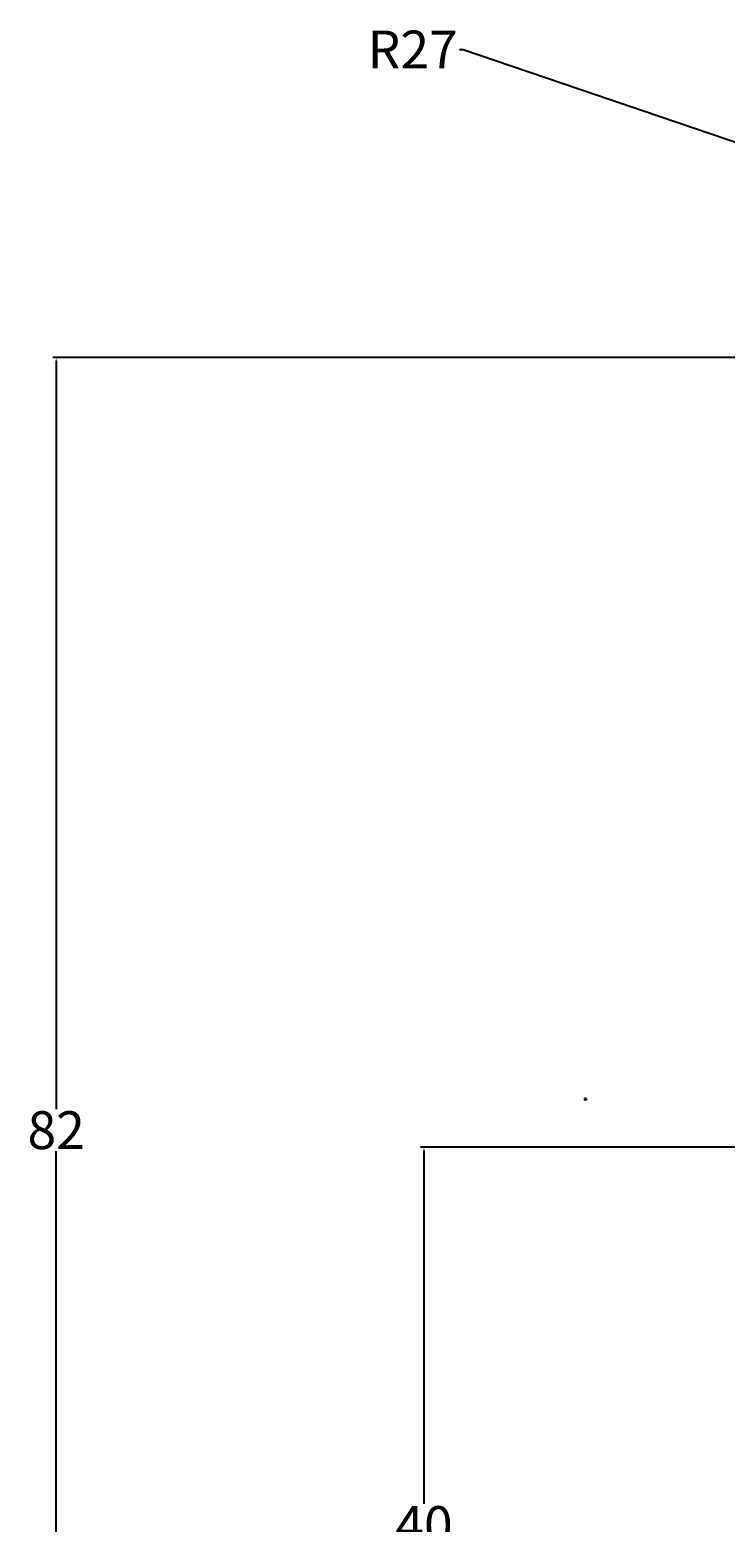
# Model space of a CAD drawing. Units: millimetres. Extents: x -60 to 113, y -37 to 126.
# Tile 6 of 17: x -60 to -23, y 27 to 106. Entities that reach past the tile are written whole.
import ezdxf

# ---------------------------------------------------------------- set-up
doc = ezdxf.new("R2010")
doc.units = ezdxf.units.MM
doc.header["$MEASUREMENT"] = 0
doc.layers.add('M-DIMS', color=2, linetype='Continuous', lineweight=25)
doc.styles.get("Standard").update_dxf_attribs({"font": 'arial.ttf'})
doc.dimstyles.get("Standard").update_dxf_attribs({"dimtxt": 0.18, "dimasz": 0.18, "dimexe": 0.18, "dimexo": 0.0625, "dimgap": 0.09, "dimtad": 0, "dimtih": 1, "dimtoh": 1, "dimdec": 4, "dimzin": 0, "dimdsep": 46, "dimtxsty": 'Standard', "dimcen": 0.09, "dimadec": 0, "dimazin": 0, "dimtfac": 1, "dimtdec": 4, "dimtofl": 0, "dimtmove": 0, "dimatfit": 3, "dimfxl": 1, "dimtolj": 1, "dimtzin": 0, "dimarcsym": 0})

# ---------------------------------------------------------------- blocks, each defined once
blk = doc.blocks.new('*D4')
at = {"layer": 'Defpoints', "color": 0, "transparency": 16777216}
for p in [(-14.94, 97.225), (10.622, 88.533)]:
    blk.add_point(p, dxfattribs=at)
at = {"layer": 'M-DIMS', "color": 0, "lineweight": -2, "transparency": 16777216}
for p, q in [((-37.421, 104.807), (-37.241, 104.807)), ((-37.241, 104.807), (-15.111, 97.283)), ((10.532, 88.533), (10.712, 88.533)), ((10.622, 88.443), (10.622, 88.623))]:
    blk.add_line(p, q, dxfattribs=at)
at = {"layer": 'M-DIMS', "color": 0, "transparency": 16777216}
blk.add_solid([(-15.101, 97.311), (-15.12, 97.254), (-14.94, 97.225)], dxfattribs=at)
at = {"layer": 'M-DIMS', "color": 0, "transparency": 16777216, "insert": (-39.9, 104.807), "char_height": 0.18, "attachment_point": 5}
blk.add_mtext('\\A1;{\\H11.11111x;R27}', dxfattribs=at)
blk = doc.blocks.new('*D6')
at = {"layer": 'Defpoints', "color": 0, "transparency": 16777216}
for p in [(-30.775, 49.351), (-0.783, 48.68)]:
    blk.add_point(p, dxfattribs=at)
at = {"layer": 'M-DIMS', "color": 0, "lineweight": -2, "transparency": 16777216}
blk.add_line((-16.661, 49.035), (-0.963, 48.684), dxfattribs=at)
at = {"layer": 'M-DIMS', "color": 0, "transparency": 16777216}
blk.add_solid([(-0.962, 48.714), (-0.963, 48.654), (-0.783, 48.68)], dxfattribs=at)
at = {"layer": 'M-DIMS', "color": 0, "transparency": 16777216, "insert": (-19.137, 49.035), "char_height": 0.18, "attachment_point": 5}
blk.add_mtext('\\A1;{\\H11.11111x;R30}', dxfattribs=at)
blk = doc.blocks.new('*D7')
at = {"layer": 'Defpoints', "color": 0, "transparency": 16777216}
for p in [(48.606, 76.822), (-30.775, 49.351)]:
    blk.add_point(p, dxfattribs=at)
at = {"layer": 'M-DIMS', "color": 0, "lineweight": -2, "transparency": 16777216}
for p, q in [((37.821, 73.09), (48.435, 76.764)), ((37.641, 73.09), (37.821, 73.09))]:
    blk.add_line(p, q, dxfattribs=at)
at = {"layer": 'M-DIMS', "color": 0, "transparency": 16777216}
blk.add_solid([(48.426, 76.792), (48.445, 76.735), (48.606, 76.822)], dxfattribs=at)
at = {"layer": 'M-DIMS', "color": 0, "transparency": 16777216, "insert": (35.165, 73.09), "char_height": 0.18, "attachment_point": 5}
blk.add_mtext('\\A1;{\\H11.11111x;R84}', dxfattribs=at)
blk = doc.blocks.new('*D12')
at = {"layer": 'Defpoints', "color": 0, "transparency": 16777216}
for p in [(10.532, 88.533), (-58.719, 6.903), (11.329, 6.903)]:
    blk.add_point(p, dxfattribs=at)
at = {"layer": 'M-DIMS', "color": 0, "lineweight": -2, "transparency": 16777216}
for p, q in [((10.47, 88.533), (-58.899, 88.533)), ((-58.719, 88.353), (-58.719, 48.829)), ((-58.719, 7.083), (-58.719, 46.607)), ((11.267, 6.903), (-58.899, 6.903))]:
    blk.add_line(p, q, dxfattribs=at)
at = {"layer": 'M-DIMS', "color": 0, "transparency": 16777216}
for points in [[(-58.749, 88.353), (-58.689, 88.353), (-58.719, 88.533)], [(-58.749, 7.083), (-58.689, 7.083), (-58.719, 6.903)]]:
    blk.add_solid(points, dxfattribs=at)
at = {"layer": 'M-DIMS', "color": 0, "transparency": 16777216, "insert": (-58.719, 47.718), "char_height": 0.18, "attachment_point": 5}
blk.add_mtext('\\A1;{\\H11.11111x;82}', dxfattribs=at)
blk = doc.blocks.new('*D13')
at = {"layer": 'Defpoints', "color": 0, "transparency": 16777216}
for p in [(37.065, 46.813), (-39.303, 6.903), (7.267, 6.903)]:
    blk.add_point(p, dxfattribs=at)
at = {"layer": 'M-DIMS', "color": 0, "lineweight": -2, "transparency": 16777216}
for p, q in [((37.002, 46.813), (-39.483, 46.813)), ((-39.303, 46.633), (-39.303, 27.969)), ((-39.303, 7.083), (-39.303, 25.747)), ((7.204, 6.903), (-39.483, 6.903))]:
    blk.add_line(p, q, dxfattribs=at)
at = {"layer": 'M-DIMS', "color": 0, "transparency": 16777216}
for points in [[(-39.333, 46.633), (-39.273, 46.633), (-39.303, 46.813)], [(-39.333, 7.083), (-39.273, 7.083), (-39.303, 6.903)]]:
    blk.add_solid(points, dxfattribs=at)
at = {"layer": 'M-DIMS', "color": 0, "transparency": 16777216, "insert": (-39.303, 26.858), "char_height": 0.18, "attachment_point": 5}
blk.add_mtext('\\A1;{\\H11.11111x;40}', dxfattribs=at)
blk = doc.blocks.new('*D24')
at = {"layer": 'Defpoints', "color": 0, "transparency": 16777216}
for p in [(48.596, 76.851), (-30.775, 49.351)]:
    blk.add_point(p, dxfattribs=at)
at = {"layer": 'M-DIMS', "color": 0, "lineweight": -2, "transparency": 16777216}
for p, q in [((96.218, 93.35), (48.766, 76.909)), ((96.398, 93.35), (96.218, 93.35)), ((-30.865, 49.351), (-30.685, 49.351)), ((-30.775, 49.261), (-30.775, 49.441))]:
    blk.add_line(p, q, dxfattribs=at)
at = {"layer": 'M-DIMS', "color": 0, "transparency": 16777216}
blk.add_solid([(48.756, 76.938), (48.776, 76.881), (48.596, 76.851)], dxfattribs=at)
at = {"layer": 'M-DIMS', "color": 0, "transparency": 16777216, "insert": (97.018, 93.35), "char_height": 0.18, "attachment_point": 5}
blk.add_mtext('\\A1;R84.0000', dxfattribs=at)
blk = doc.blocks.new('*D25')
at = {"layer": 'Defpoints', "color": 0, "transparency": 16777216}
for p in [(-30.775, 49.351), (-0.782, 48.7)]:
    blk.add_point(p, dxfattribs=at)
at = {"layer": 'M-DIMS', "color": 0, "lineweight": -2, "transparency": 16777216}
for p, q in [((-30.865, 49.351), (-30.685, 49.351)), ((-30.775, 49.261), (-30.775, 49.441)), ((17.214, 48.309), (-0.602, 48.696))]:
    blk.add_line(p, q, dxfattribs=at)
at = {"layer": 'M-DIMS', "color": 0, "transparency": 16777216}
blk.add_solid([(-0.602, 48.726), (-0.603, 48.666), (-0.782, 48.7)], dxfattribs=at)
at = {"layer": 'M-DIMS', "color": 0, "transparency": 16777216, "insert": (17.833, 48.309), "char_height": 0.18, "attachment_point": 5}
blk.add_mtext('\\A1;R30.0000', dxfattribs=at)

msp = doc.modelspace()

# ---------------------------------------------------------------- dimensions: what is measured, and where the dimension line sits
at = {"layer": 'M-DIMS'}
for center, mpoint, text, picture, middle in [((10.62227, 88.53289), (-14.94042, 97.22479), '{\\H11.11111x;R27}', '*D4', (-39.9004, 104.80746)), ((-30.77517, 49.3506), (48.60556, 76.82239), '{\\H11.11111x;R84}', '*D7', (35.16548, 73.09007)), ((-30.77517, 49.3506), (-0.78268, 48.6796), '{\\H11.11111x;R30}', '*D6', (-16.66078, 49.03483))]:
    dim = msp.add_radius_dim(center=center, mpoint=mpoint, text=text, dimstyle='Standard', override={"dimclrd": 0, "dimclre": 0, "dimclrt": 0}, dxfattribs=at)
    dim.commit()
    dim.dimension.update_dxf_attribs({"geometry": picture, "text_midpoint": middle, "dimtype": 164})
for mpoint, picture, middle in [((48.59582, 76.85052), '*D24', (97.01779, 93.35047)), ((-0.78224, 48.69961), '*D25', (17.21352, 48.30902))]:
    dim = msp.add_radius_dim(center=(-30.77517, 49.3506), mpoint=mpoint, dimstyle='Standard', override={"dimdec": 4, "dimlfac": 1, "dimrnd": 0, "dimzin": 0, "dimdsep": 46, "dimlunit": 2}, dxfattribs=at)
    dim.commit()
    dim.dimension.update_dxf_attribs({"geometry": picture, "text_midpoint": middle, "dimtype": 164})
for base, p1, p2, text, picture, middle in [((-58.71857, 6.9027), (10.53227, 88.53289), (11.32938, 6.9027), '{\\H11.11111x;82}', '*D12', (-58.71857, 47.71779)), ((-39.30316, 6.9027), (37.06463, 46.81263), (7.26659, 6.9027), '{\\H11.11111x;40}', '*D13', (-39.30316, 26.85766))]:
    dim = msp.add_linear_dim(base=base, p1=p1, p2=p2, angle=90, text=text, dimstyle='Standard', override={"dimclrd": 0, "dimclre": 0, "dimclrt": 0}, dxfattribs=at)
    dim.commit()
    dim.dimension.update_dxf_attribs({"geometry": picture, "text_midpoint": middle})

doc.saveas('drawing.dxf')
